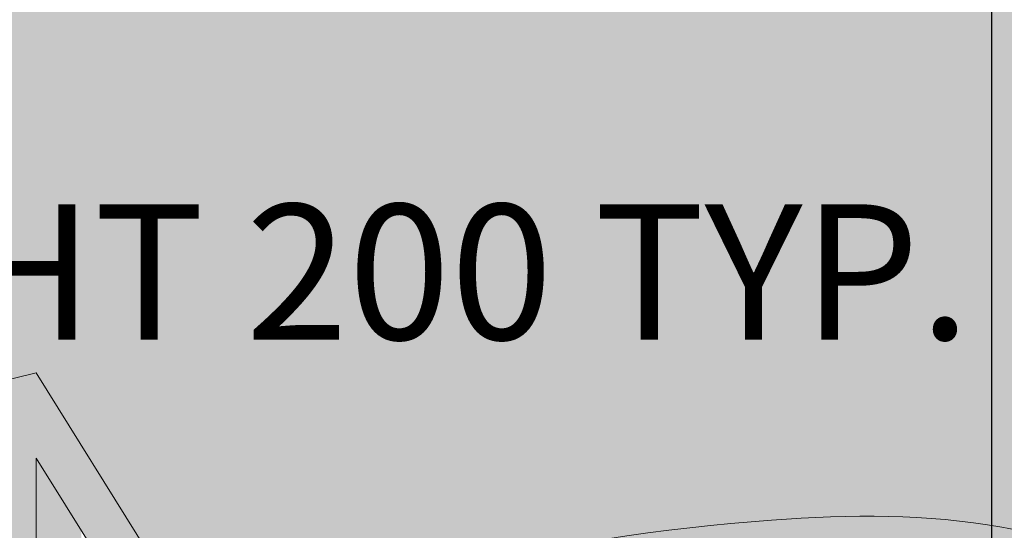
# Model space of a CAD drawing. Units: millimetres. Extents: x 11032 to 26788, y 3406 to 24505.
# Tile 56 of 78: x 15266 to 16358, y 16877 to 17443. Entities that reach past the tile are written whole.
import ezdxf

# ---------------------------------------------------------------- set-up
doc = ezdxf.new("R2010")
doc.units = ezdxf.units.MM
doc.header["$MEASUREMENT"] = 0
for name, color, linetype, lineweight in [('A-ANNO-DIMS', 2, 'Continuous', 18), ('A-GLAZ', 250, 'Continuous', 20), ('A-ROOF', 7, 'Continuous', 30), ('E-LITE', 7, 'Continuous', 18), ('E-LITE-PATT', 7, 'Continuous', 13)]:
    doc.layers.add(name, color=color, linetype=linetype, lineweight=lineweight)
for name, color, linetype, lineweight, true_color in [('A-GLAZ-FRAM-PATT', 250, 'Continuous', 13, 0x262627), ('A-ROOF-PATT', 9, 'Continuous', 13, 0xc7c8ca), ('A-WALL-INTR-PATT', 251, 'Continuous', 13, 0x6c6b6a)]:
    doc.layers.add(name, color=color, linetype=linetype, lineweight=lineweight, true_color=true_color)
doc.styles.get("Standard").update_dxf_attribs({"font": 'arial.ttf'})
doc.dimstyles.get("Standard").update_dxf_attribs({"dimtxt": 150, "dimasz": 100, "dimexe": 10, "dimexo": 5, "dimgap": 5, "dimtad": 0, "dimtih": 1, "dimtoh": 1, "dimdec": 0, "dimzin": 0, "dimdsep": 46, "dimtxsty": 'Standard', "dimcen": 0.09, "dimadec": 0, "dimazin": 0, "dimtfac": 1, "dimtdec": 0, "dimtofl": 0, "dimtmove": 0, "dimatfit": 3, "dimfxl": 1, "dimtolj": 1, "dimtzin": 0, "dimarcsym": 0})

# ---------------------------------------------------------------- blocks, each defined once
blk = doc.blocks.new('*D24')
at = {"layer": 'A-ANNO-DIMS', "color": 0, "lineweight": -2, "transparency": 16777216}
for p, q in [((13310.2, 17138), (13310.2, 17173)), ((13510.2, 17138), (13510.2, 17173)), ((13210.2, 17163), (13110.2, 17163)), ((13610.2, 17163), (13710.2, 17163))]:
    blk.add_line(p, q, dxfattribs=at)
at = {"layer": 'A-ANNO-DIMS', "color": 0, "transparency": 16777216}
for points in [[(13210.2, 17179.6), (13210.2, 17146.3), (13310.2, 17163)], [(13610.2, 17179.6), (13610.2, 17146.3), (13510.2, 17163)]]:
    blk.add_solid(points, dxfattribs=at)
at = {"layer": 'Defpoints', "color": 0, "transparency": 16777216}
for p in [(13510.2, 17163), (13310.2, 17133), (13510.2, 17133)]:
    blk.add_point(p, dxfattribs=at)
at = {"layer": 'A-ANNO-DIMS', "color": 0, "transparency": 16777216, "insert": (15077.8, 17163), "char_height": 150, "attachment_point": 5}
blk.add_mtext('\\A1;RECESSED LIGHT 200 TYP.', dxfattribs=at)
blk = doc.blocks.new('*D36')
at = {"layer": 'A-ANNO-DIMS', "color": 0, "lineweight": -2, "transparency": 16777216}
for p, q in [((12301.3, 17115.9), (12301.3, 24416.9)), ((25397.4, 4466.4), (25397.4, 24416.9)), ((12401.3, 24406.9), (18569.2, 24406.9)), ((25297.4, 24406.9), (19129.5, 24406.9))]:
    blk.add_line(p, q, dxfattribs=at)
at = {"layer": 'A-ANNO-DIMS', "color": 0, "transparency": 16777216}
for points in [[(12401.3, 24423.5), (12401.3, 24390.2), (12301.3, 24406.9)], [(25297.4, 24423.5), (25297.4, 24390.2), (25397.4, 24406.9)]]:
    blk.add_solid(points, dxfattribs=at)
at = {"layer": 'Defpoints', "color": 0, "transparency": 16777216}
for p in [(25397.4, 24406.9), (12301.3, 17110.9), (25397.4, 4461.4)]:
    blk.add_point(p, dxfattribs=at)
at = {"layer": 'A-ANNO-DIMS', "color": 0, "transparency": 16777216, "insert": (18849.3, 24406.9), "char_height": 150, "attachment_point": 5}
blk.add_mtext('\\A1;13096', dxfattribs=at)
blk = doc.blocks.new('*D37')
at = {"layer": 'A-ANNO-DIMS', "color": 0, "lineweight": -2, "transparency": 16777216}
for p, q in [((18087.7, 23450.4), (11334.8, 23450.4)), ((11344.8, 23350.4), (11344.8, 14037.5)), ((11344.8, 4561.4), (11344.8, 13874.3)), ((12927.7, 4461.4), (11334.8, 4461.4))]:
    blk.add_line(p, q, dxfattribs=at)
at = {"layer": 'A-ANNO-DIMS', "color": 0, "transparency": 16777216}
for points in [[(11328.1, 23350.4), (11361.4, 23350.4), (11344.8, 23450.4)], [(11328.1, 4561.4), (11361.4, 4561.4), (11344.8, 4461.4)]]:
    blk.add_solid(points, dxfattribs=at)
at = {"layer": 'Defpoints', "color": 0, "transparency": 16777216}
for p in [(11344.8, 23450.4), (18092.7, 23450.4), (12932.7, 4461.4)]:
    blk.add_point(p, dxfattribs=at)
at = {"layer": 'A-ANNO-DIMS', "color": 0, "transparency": 16777216, "insert": (11344.8, 13955.9), "char_height": 150, "attachment_point": 5}
blk.add_mtext('\\A1;18989', dxfattribs=at)
blk = doc.blocks.new('*D45')
at = {"layer": 'A-ANNO-DIMS', "color": 0, "lineweight": -2, "transparency": 16777216}
for p, q in [((13792.4, 18518.9), (26363.9, 18518.9)), ((26353.9, 18418.9), (26353.9, 17450.3)), ((26353.9, 16318.4), (26353.9, 17287)), ((22902.4, 16218.4), (26363.9, 16218.4))]:
    blk.add_line(p, q, dxfattribs=at)
at = {"layer": 'A-ANNO-DIMS', "color": 0, "transparency": 16777216}
for points in [[(26337.2, 18418.9), (26370.6, 18418.9), (26353.9, 18518.9)], [(26337.2, 16318.4), (26370.6, 16318.4), (26353.9, 16218.4)]]:
    blk.add_solid(points, dxfattribs=at)
at = {"layer": 'Defpoints', "color": 0, "transparency": 16777216}
for p in [(13787.4, 18518.9), (26353.9, 18518.9), (22897.4, 16218.4)]:
    blk.add_point(p, dxfattribs=at)
at = {"layer": 'A-ANNO-DIMS', "color": 0, "transparency": 16777216, "insert": (26353.9, 17368.7), "char_height": 150, "attachment_point": 5}
blk.add_mtext('\\A1;2300.5', dxfattribs=at)
blk = doc.blocks.new('*D57')
at = {"layer": 'A-ANNO-DIMS', "color": 0, "lineweight": -2, "transparency": 16777216}
for p, q in [((14994.7, 7266.4), (14994.7, 24416.9)), ((20894.7, 7266.4), (20894.7, 24416.9)), ((15094.7, 24406.9), (17716, 24406.9)), ((20794.7, 24406.9), (18173.4, 24406.9))]:
    blk.add_line(p, q, dxfattribs=at)
at = {"layer": 'A-ANNO-DIMS', "color": 0, "transparency": 16777216}
for points in [[(15094.7, 24423.5), (15094.7, 24390.2), (14994.7, 24406.9)], [(20794.7, 24423.5), (20794.7, 24390.2), (20894.7, 24406.9)]]:
    blk.add_solid(points, dxfattribs=at)
at = {"layer": 'Defpoints', "color": 0, "transparency": 16777216}
for p in [(20894.7, 24406.9), (14994.7, 7261.4), (20894.7, 7261.4)]:
    blk.add_point(p, dxfattribs=at)
at = {"layer": 'A-ANNO-DIMS', "color": 0, "transparency": 16777216, "insert": (17944.7, 24406.9), "char_height": 150, "attachment_point": 5}
blk.add_mtext('\\A1;5900', dxfattribs=at)
blk = doc.blocks.new('*D60')
at = {"layer": 'A-ANNO-DIMS', "color": 0, "lineweight": -2, "transparency": 16777216}
for p, q in [((14994.7, 7266.4), (14994.7, 24416.9)), ((16344.7, 7266.4), (16344.7, 24416.9)), ((15094.7, 24406.9), (15448, 24406.9)), ((16244.7, 24406.9), (15891.4, 24406.9))]:
    blk.add_line(p, q, dxfattribs=at)
at = {"layer": 'A-ANNO-DIMS', "color": 0, "transparency": 16777216}
for points in [[(15094.7, 24423.5), (15094.7, 24390.2), (14994.7, 24406.9)], [(16244.7, 24423.5), (16244.7, 24390.2), (16344.7, 24406.9)]]:
    blk.add_solid(points, dxfattribs=at)
at = {"layer": 'Defpoints', "color": 0, "transparency": 16777216}
for p in [(16344.7, 24406.9), (14994.7, 7261.4), (16344.7, 7261.4)]:
    blk.add_point(p, dxfattribs=at)
at = {"layer": 'A-ANNO-DIMS', "color": 0, "transparency": 16777216, "insert": (15669.7, 24406.9), "char_height": 150, "attachment_point": 5}
blk.add_mtext('\\A1;1350', dxfattribs=at)

msp = doc.modelspace()

# ---------------------------------------------------------------- hatches: boundary and pattern name
at = {"layer": 'A-GLAZ-FRAM-PATT'}
h = msp.add_hatch(color=256, dxfattribs=at)
edge = h.paths.add_edge_path()
edge.add_line((15284.393, 17051.32), (15084.393, 17001.32))
edge.add_line((15084.393, 17001.32), (15084.393, 15951.32))
edge.add_spline(control_points=[(15084.393, 15951.32), (15157.266, 15924.219), (15224.458, 15897.808), (15284.393, 15870.289)], knot_values=[511.94901044, 511.94901044, 511.94901044, 511.94901044, 697.37159794, 697.37159794, 697.37159794, 697.37159794], degree=3, periodic=0)
edge.add_line((15284.393, 15870.289), (15284.393, 17051.32))
edge = h.paths.add_edge_path()
edge.add_line((15659.393, 16354.387), (15459.393, 16675.629))
edge.add_line((15459.393, 16675.629), (15459.393, 15771.505))
edge.add_spline(control_points=[(15459.393, 15771.505), (15501.891, 15741.568), (15571.096, 15682.692), (15632.72, 15612.509), (15659.393, 15578.299)], knot_values=[905.064582, 905.064582, 905.064582, 905.064582, 1079.4682707, 1223.15843531, 1223.15843531, 1223.15843531, 1223.15843531], degree=3, periodic=0)
edge.add_line((15659.393, 15578.299), (15659.393, 16354.387))
h.paths.add_polyline_path([(15284.393, 17051.32), (15284.393, 16956.717), (15784.393, 16153.61), (15784.393, 16248.213)])
at = {"layer": 'A-ROOF-PATT'}
h = msp.add_hatch(color=256, dxfattribs=at)
edge = h.paths.add_edge_path()
edge.add_spline(control_points=[(17532.827, 17324.837), (17391.335, 17349.016), (16840.872, 17494.912), (16080.055, 18069.544), (14738.803, 18299.641), (13382.429, 18838.336), (12580.532, 17870.207), (12430.422, 17563.822)], knot_values=[2977.60279446, 2977.60279446, 2977.60279446, 2977.60279446, 3438.18406011, 4811.64630219, 5622.86754827, 7588.02881883, 8560.66857913, 8560.66857913, 8560.66857913, 8560.66857913], degree=3, periodic=0)
edge.add_spline(control_points=[(12430.422, 17563.822), (12437.904, 17573.36), (12445.386, 17582.899), (12452.869, 17592.437), (12452.869, 17592.438), (12452.869, 17592.438), (12452.869, 17592.438)], knot_values=[1408.56413798, 1408.56413798, 1408.56413798, 1408.56413798, 1444.85989, 1444.85989, 1444.85989, 1444.86011829, 1444.86011829, 1444.86011829, 1444.86011829], degree=3, periodic=0)
edge.add_spline(control_points=[(12452.869, 17592.438), (12555.432, 17723.185), (12736.557, 17929.686), (13044.86, 18114.643), (13219.943, 18189.644), (13299.92, 18220.646)], knot_values=[339.31824597, 339.31824597, 339.31824597, 339.31824597, 836.83499673, 1151.25129334, 1408.56413798, 1408.56413798, 1408.56413798, 1408.56413798], degree=3, periodic=0)
edge.add_spline(control_points=[(13299.92, 18220.646), (13299.998, 18220.689), (13300.077, 18220.732), (13319.738, 18231.488), (13339.24, 18241.402), (13388.645, 18264.703), (13418.466, 18277.069), (13478.019, 18298.648), (13507.751, 18307.861), (13544.561, 18317.488), (13551.584, 18319.245), (13558.612, 18320.924)], knot_values=[3783.89509717, 3783.89509717, 3783.89509717, 3783.89509717, 3784.1737101, 3784.1737101, 3853.4666747, 3853.4666747, 3960.24019172, 3960.24019172, 4067.01370874, 4067.01370874, 4092.17446487, 4092.17446487, 4092.17446487, 4092.17446487], degree=3, periodic=0)
edge.add_spline(control_points=[(13558.612, 18320.924), (13581.407, 18326.373), (13604.25, 18331.007), (13657.184, 18339.957), (13687.338, 18343.732), (13748.098, 18348.892), (13778.704, 18350.276), (13840.46, 18350.833), (13871.609, 18350.005), (13934.496, 18346.313), (13966.232, 18343.449), (14030.297, 18335.871), (14062.625, 18331.158), (14127.853, 18320.088), (14160.753, 18313.73), (14241.357, 18296.556), (14289.343, 18284.997), (14386.31, 18259.688), (14435.291, 18245.941), (14534.161, 18217.034), (14584.049, 18201.875), (14684.682, 18170.964), (14735.427, 18155.212), (14837.763, 18123.971), (14889.354, 18108.482), (14954.971, 18089.677), (14968.586, 18085.823), (14992.391, 18079.184), (15002.566, 18076.376), (15021.739, 18071.153), (15030.731, 18068.729), (15047.707, 18064.21), (15055.694, 18062.106), (15079.815, 18055.825), (15095.905, 18051.728), (15143.966, 18039.717), (15175.729, 18032.084), (15254.84, 18013.501), (15301.798, 18002.866), (15394.186, 17981.845), (15439.615, 17971.459), (15528.833, 17950.135), (15572.62, 17939.197), (15658.477, 17916.021), (15700.546, 17903.785), (15753.633, 17886.734), (15765.446, 17882.835), (15786.574, 17875.653), (15795.915, 17872.404), (15810.108, 17867.349), (15814.99, 17865.588), (15824.736, 17862.029), (15829.611, 17860.226), (15844.241, 17854.75), (15854.002, 17851.008), (15883.312, 17839.521), (15902.885, 17831.512), (15966.355, 17804.548), (16010.39, 17784.302), (16098.838, 17741.267), (16143.25, 17718.478), (16232.497, 17671.098), (16277.332, 17646.507), (16367.515, 17596.295), (16412.862, 17570.676), (16504.202, 17519.209), (16550.194, 17493.362), (16643.009, 17442.263), (16689.831, 17417.011), (16756.517, 17382.472), (16775.937, 17372.58), (16795.455, 17362.84)], knot_values=[4092.17446487, 4092.17446487, 4092.17446487, 4092.17446487, 4173.78722577, 4173.78722577, 4280.56074279, 4280.56074279, 4387.33425981, 4387.33425981, 4494.10777683, 4494.10777683, 4600.88129386, 4600.88129386, 4707.65481088, 4707.65481088, 4814.4283279, 4814.4283279, 4967.12624049, 4967.12624049, 5119.82415308, 5119.82415308, 5272.52206566, 5272.52206566, 5425.21997825, 5425.21997825, 5577.91789084, 5577.91789084, 5617.78533194, 5617.78533194, 5647.46484794, 5647.46484794, 5673.61102495, 5673.61102495, 5696.74760695, 5696.74760695, 5743.68189033, 5743.68189033, 5837.55045709, 5837.55045709, 5979.72610459, 5979.72610459, 6121.90175208, 6121.90175208, 6264.07739957, 6264.07739957, 6406.25304706, 6406.25304706, 6447.25858494, 6447.25858494, 6480.04208821, 6480.04208821, 6497.30770621, 6497.30770621, 6514.5733242, 6514.5733242, 6549.10456019, 6549.10456019, 6618.16703217, 6618.16703217, 6772.66101707, 6772.66101707, 6927.15500198, 6927.15500198, 7081.64898689, 7081.64898689, 7236.1429718, 7236.1429718, 7390.6369567, 7390.6369567, 7545.13094161, 7545.13094161, 7608.19928683, 7608.19928683, 7608.19928683, 7608.19928683], degree=3, periodic=0)
edge.add_spline(control_points=[(16795.455, 17362.84), (16814.335, 17349.456), (16832.897, 17336.263), (16873.225, 17307.197), (16894.778, 17291.386), (16936.221, 17259.941), (16956.11, 17244.308), (16993.863, 17213.094), (17011.726, 17197.514), (17041.993, 17169.265), (17054.791, 17156.601), (17078.762, 17131.225), (17089.933, 17118.516), (17110.618, 17092.991), (17120.131, 17080.178), (17130.17, 17065.264), (17131.487, 17063.277), (17133.77, 17059.776), (17134.746, 17058.261), (17136.69, 17055.205), (17137.657, 17053.668), (17140.539, 17049.025), (17142.438, 17045.89), (17148.068, 17036.367), (17151.732, 17029.859), (17163.03, 17008.788), (17170.335, 16993.646), (17184.087, 16961.978), (17190.534, 16945.453), (17202.562, 16911.165), (17208.142, 16893.402), (17218.448, 16856.821), (17223.173, 16838.003), (17231.801, 16799.51), (17235.705, 16779.837), (17241.533, 16746.739), (17243.676, 16733.5), (17247.718, 16706.37), (17249.608, 16692.472), (17252.066, 16672.69), (17252.761, 16666.875), (17254.1, 16655.226), (17254.744, 16649.4), (17256.596, 16631.917), (17257.727, 16620.254), (17260.823, 16585.238), (17262.489, 16561.858), (17266.551, 16488.654), (17267.658, 16438.661), (17267.349, 16375.228), (17267.193, 16362.07), (17266.95, 16348.891)], knot_values=[15.11304723, 15.11304723, 15.11304723, 15.11304723, 82.69951457, 82.69951457, 165.39902914, 165.39902914, 248.09854371, 248.09854371, 330.79805828, 330.79805828, 397.94194582, 397.94194582, 465.08583335, 465.08583335, 532.22972088, 532.22972088, 542.53374101, 542.53374101, 550.35681582, 550.35681582, 558.17989062, 558.17989062, 573.82604024, 573.82604024, 605.11833946, 605.11833946, 672.76406143, 672.76406143, 740.4097834, 740.4097834, 808.05550537, 808.05550537, 875.70122735, 875.70122735, 943.34694932, 943.34694932, 987.66134917, 987.66134917, 1033.41216123, 1033.41216123, 1052.38508762, 1052.38508762, 1071.35801402, 1071.35801402, 1109.30386682, 1109.30386682, 1185.19557241, 1185.19557241, 1346.44190265, 1346.44190265, 1388.55866312, 1388.55866312, 1388.55866312, 1388.55866312], degree=3, periodic=0)
edge.add_spline(control_points=[(17266.95, 16348.891), (17266.95, 16348.891), (17266.95, 16348.891), (17266.95, 16348.891), (17253.182, 15602.417), (17239.414, 14855.943), (17225.646, 14109.469)], knot_values=[1388.55866312, 1388.55866312, 1388.55866312, 1388.55866312, 1388.55896543, 1388.55896543, 1388.55896543, 3774.07676609, 3774.07676609, 3774.07676609, 3774.07676609], degree=3, periodic=0)
edge.add_spline(control_points=[(17225.646, 14109.469), (17226.198, 14109.827), (17226.748, 14110.185), (17242.065, 14120.191), (17255.956, 14130.116), (17274.422, 14144.286), (17279.609, 14148.386), (17284.686, 14152.511)], knot_values=[1926.3423968, 1926.3423968, 1926.3423968, 1926.3423968, 1927.31672898, 1927.31672898, 1953.51217613, 1953.51217613, 1964.07323478, 1964.07323478, 1964.07323478, 1964.07323478], degree=3, periodic=0)
edge.add_spline(control_points=[(17284.686, 14152.511), (17315.791, 14194.761), (17384.413, 14446.273), (17407.128, 14793.401), (17407.093, 15295.84), (17423.274, 15626.362), (17415.601, 15782.507)], knot_values=[0, 0, 0, 0, 163.25546741, 619.22967667, 1171.8624483, 1621.63555623, 1621.63555623, 1621.63555623, 1621.63555623], degree=3, periodic=0)
edge.add_spline(control_points=[(17415.601, 15782.507), (17438.21, 16077.57), (17410.495, 16533.484), (17390.893, 17030.649), (17301.082, 17169.349)], knot_values=[543.97847526, 543.97847526, 543.97847526, 543.97847526, 1452.98527668, 1960.01149261, 1960.01149261, 1960.01149261, 1960.01149261], degree=3, periodic=0)
edge.add_spline(control_points=[(17301.082, 17169.349), (17346.58, 17157.64), (17392.235, 17147.336), (17467.161, 17132.609), (17496.336, 17127.412), (17525.58, 17122.709)], knot_values=[8131.59393903, 8131.59393903, 8131.59393903, 8131.59393903, 8269.73492727, 8269.73492727, 8357.5016646, 8357.5016646, 8357.5016646, 8357.5016646], degree=3, periodic=0)
edge.add_line((17525.58, 17122.709), (17532.827, 17324.837))
edge = h.paths.add_edge_path(flags=17)
edge.add_spline(control_points=[(13340.537, 14602.706), (13316.172, 14726.456), (13323.666, 14932.342), (13637.836, 15081.117), (13863.248, 15171.051), (14002.1, 15224.503), (14058.539, 15244.876)], knot_values=[680.89318617, 680.89318617, 680.89318617, 680.89318617, 1033.47282894, 1337.40083264, 1604.72142636, 1784.29447217, 1784.29447217, 1784.29447217, 1784.29447217], degree=3, periodic=0)
edge.add_spline(control_points=[(14058.539, 15244.876), (14058.289, 15275.236), (14057.634, 15305.434), (14055.312, 15376.527), (14053.359, 15417.248), (14048.642, 15497.048), (14045.89, 15536.143), (14042.888, 15574.619)], knot_values=[6573.10654186, 6573.10654186, 6573.10654186, 6573.10654186, 6636.73300118, 6636.73300118, 6723.88905466, 6723.88905466, 6809.63287714, 6809.63287714, 6809.63287714, 6809.63287714], degree=3, periodic=0)
edge.add_spline(control_points=[(14042.888, 15574.619), (13546.54, 15403.221), (13074.735, 15143.241), (13277.36, 14695.339), (13340.537, 14602.706)], knot_values=[503.79257829, 503.79257829, 503.79257829, 503.79257829, 1728.17876056, 2051.34843998, 2051.34843998, 2051.34843998, 2051.34843998], degree=3, periodic=0)
h = msp.add_hatch(color=256, dxfattribs=at)
h.set_gradient(color1=(254, 234, 185), color2=(254, 204, 102), name='HEMISPHERICAL')
edge = h.paths.add_edge_path()
edge.add_line((15084.393, 17001.32), (15284.393, 17051.32))
edge.add_line((15284.393, 17051.32), (15470.537, 16752.334))
edge.add_spline(control_points=[(15470.537, 16752.334), (15683.311, 16831.508), (16106.827, 16912.335), (16625.609, 16876.997), (17083.498, 16357.78), (17257.801, 16180.113)], knot_values=[0, 0, 0, 0, 655.29363337, 1252.01578382, 1989.61628586, 1989.61628586, 1989.61628586, 1989.61628586], degree=3, periodic=0)
edge.add_spline(control_points=[(17257.801, 16180.113), (17260.851, 16236.372), (17263.9, 16292.632), (17266.95, 16348.891)], knot_values=[1132.9967717, 1132.9967717, 1132.9967717, 1132.9967717, 1198.04642249, 1198.04642249, 1198.04642249, 1198.04642249], degree=3, periodic=0)
edge.add_spline(control_points=[(17266.95, 16348.891), (17267.193, 16362.07), (17267.349, 16375.228), (17267.658, 16438.661), (17266.551, 16488.654), (17262.489, 16561.858), (17260.823, 16585.238), (17257.727, 16620.254), (17256.596, 16631.917), (17254.744, 16649.4), (17254.1, 16655.226), (17252.761, 16666.875), (17252.066, 16672.69), (17249.608, 16692.472), (17247.718, 16706.37), (17243.676, 16733.5), (17241.533, 16746.739), (17235.705, 16779.837), (17231.801, 16799.51), (17223.173, 16838.003), (17218.448, 16856.821), (17208.142, 16893.402), (17202.562, 16911.165), (17190.534, 16945.453), (17184.087, 16961.978), (17170.335, 16993.646), (17163.03, 17008.788), (17151.732, 17029.859), (17148.068, 17036.367), (17142.438, 17045.89), (17140.539, 17049.025), (17137.657, 17053.668), (17136.69, 17055.205), (17134.746, 17058.261), (17133.77, 17059.776), (17131.487, 17063.277), (17130.17, 17065.264), (17120.131, 17080.178), (17110.618, 17092.991), (17089.933, 17118.516), (17078.762, 17131.225), (17054.791, 17156.601), (17041.993, 17169.265), (17011.726, 17197.514), (16993.863, 17213.094), (16956.11, 17244.308), (16936.221, 17259.941), (16894.778, 17291.386), (16873.225, 17307.197), (16832.897, 17336.263), (16814.335, 17349.456), (16795.455, 17362.84)], knot_values=[15.11304723, 15.11304723, 15.11304723, 15.11304723, 57.2298077, 57.2298077, 218.47613793, 218.47613793, 294.36784353, 294.36784353, 332.31369632, 332.31369632, 351.28662272, 351.28662272, 370.25954912, 370.25954912, 416.01036118, 416.01036118, 460.32476103, 460.32476103, 527.970483, 527.970483, 595.61620497, 595.61620497, 663.26192694, 663.26192694, 730.90764891, 730.90764891, 798.55337089, 798.55337089, 829.84567011, 829.84567011, 845.49181972, 845.49181972, 853.31489453, 853.31489453, 861.13796933, 861.13796933, 871.44198947, 871.44198947, 938.585877, 938.585877, 1005.72976453, 1005.72976453, 1072.87365206, 1072.87365206, 1155.57316663, 1155.57316663, 1238.2726812, 1238.2726812, 1320.97219578, 1320.97219578, 1388.55866312, 1388.55866312, 1388.55866312, 1388.55866312], degree=3, periodic=0)
edge.add_spline(control_points=[(16795.455, 17362.84), (16775.937, 17372.58), (16756.517, 17382.472), (16689.831, 17417.011), (16643.009, 17442.263), (16550.194, 17493.362), (16504.202, 17519.209), (16412.862, 17570.676), (16367.515, 17596.295), (16277.332, 17646.507), (16232.497, 17671.098), (16143.25, 17718.478), (16098.838, 17741.267), (16010.39, 17784.302), (15966.355, 17804.548), (15902.885, 17831.512), (15883.312, 17839.521), (15854.002, 17851.008), (15844.241, 17854.75), (15829.611, 17860.226), (15824.736, 17862.029), (15814.99, 17865.588), (15810.108, 17867.349), (15795.915, 17872.404), (15786.574, 17875.653), (15765.446, 17882.835), (15753.633, 17886.734), (15700.546, 17903.785), (15658.477, 17916.021), (15572.62, 17939.197), (15528.833, 17950.135), (15439.615, 17971.459), (15394.186, 17981.845), (15301.798, 18002.866), (15254.84, 18013.501), (15175.729, 18032.084), (15143.966, 18039.717), (15095.905, 18051.728), (15079.815, 18055.825), (15055.694, 18062.106), (15047.707, 18064.21), (15030.731, 18068.729), (15021.739, 18071.153), (15002.566, 18076.376), (14992.391, 18079.184), (14968.586, 18085.823), (14954.971, 18089.677), (14889.354, 18108.482), (14837.763, 18123.971), (14735.427, 18155.212), (14684.682, 18170.964), (14584.049, 18201.875), (14534.161, 18217.034), (14435.291, 18245.941), (14386.31, 18259.688), (14289.343, 18284.997), (14241.357, 18296.556), (14160.753, 18313.73), (14127.853, 18320.088), (14062.625, 18331.158), (14030.297, 18335.871), (13966.232, 18343.449), (13934.496, 18346.313), (13871.609, 18350.005), (13840.46, 18350.833), (13778.704, 18350.276), (13748.098, 18348.892), (13687.338, 18343.732), (13657.184, 18339.957), (13604.25, 18331.007), (13581.407, 18326.373), (13558.612, 18320.924)], knot_values=[4092.17446487, 4092.17446487, 4092.17446487, 4092.17446487, 4155.24281009, 4155.24281009, 4309.736795, 4309.736795, 4464.2307799, 4464.2307799, 4618.72476481, 4618.72476481, 4773.21874972, 4773.21874972, 4927.71273463, 4927.71273463, 5082.20671953, 5082.20671953, 5151.26919151, 5151.26919151, 5185.8004275, 5185.8004275, 5203.0660455, 5203.0660455, 5220.33166349, 5220.33166349, 5253.11516676, 5253.11516676, 5294.12070464, 5294.12070464, 5436.29635213, 5436.29635213, 5578.47199962, 5578.47199962, 5720.64764711, 5720.64764711, 5862.82329461, 5862.82329461, 5956.69186137, 5956.69186137, 6003.62614475, 6003.62614475, 6026.76272675, 6026.76272675, 6052.90890376, 6052.90890376, 6082.58841976, 6082.58841976, 6122.45586086, 6122.45586086, 6275.15377345, 6275.15377345, 6427.85168604, 6427.85168604, 6580.54959862, 6580.54959862, 6733.24751121, 6733.24751121, 6885.9454238, 6885.9454238, 6992.71894082, 6992.71894082, 7099.49245784, 7099.49245784, 7206.26597487, 7206.26597487, 7313.03949189, 7313.03949189, 7419.81300891, 7419.81300891, 7526.58652593, 7526.58652593, 7608.19928683, 7608.19928683, 7608.19928683, 7608.19928683], degree=3, periodic=0)
edge.add_spline(control_points=[(13558.612, 18320.924), (13472.381, 18287.498), (13386.15, 18254.072), (13299.92, 18220.646), (13299.92, 18220.646), (13299.92, 18220.646), (13299.92, 18220.646)], knot_values=[61.88324569, 61.88324569, 61.88324569, 61.88324569, 339.3179746, 339.3179746, 339.3179746, 339.31824597, 339.31824597, 339.31824597, 339.31824597], degree=3, periodic=0)
edge.add_spline(control_points=[(13299.92, 18220.646), (13219.943, 18189.644), (13044.86, 18114.643), (12736.557, 17929.686), (12555.432, 17723.185), (12452.869, 17592.438)], knot_values=[339.31824597, 339.31824597, 339.31824597, 339.31824597, 596.63109061, 911.04738723, 1408.56413798, 1408.56413798, 1408.56413798, 1408.56413798], degree=3, periodic=0)
edge.add_spline(control_points=[(12452.869, 17592.438), (12452.869, 17592.438), (12452.869, 17592.438), (12452.869, 17592.437), (12445.386, 17582.899), (12437.904, 17573.36), (12430.422, 17563.822)], knot_values=[1408.56413798, 1408.56413798, 1408.56413798, 1408.56413798, 1408.56436627, 1408.56436627, 1408.56436627, 1444.86011829, 1444.86011829, 1444.86011829, 1444.86011829], degree=3, periodic=0)
edge.add_spline(control_points=[(12430.422, 17563.822), (12373.797, 17448.248), (12157.302, 16836.764), (12751.985, 16393.69), (13424.325, 15907.903), (14042.888, 15574.619)], knot_values=[0, 0, 0, 0, 366.89930338, 1975.59410824, 2977.60279446, 2977.60279446, 2977.60279446, 2977.60279446], degree=3, periodic=0)
edge.add_spline(control_points=[(14042.888, 15574.619), (14042.839, 15575.252), (14042.789, 15575.886), (14039.681, 15615.607), (14036.366, 15654.052), (14029.551, 15729.305), (14026.05, 15766.114), (14019.175, 15837.686), (14015.8, 15872.45), (13903.823, 16338.596)], knot_values=[6310.22615039, 6310.22615039, 6310.22615039, 6310.22615039, 6311.63838141, 6311.63838141, 6398.79443489, 6398.79443489, 6485.95048837, 6485.95048837, 6573.10654186, 6573.10654186, 6573.10654186, 6573.10654186], degree=3, periodic=0)
edge.add_spline(control_points=[(13903.823, 16338.596), (14237.315, 16236.889), (14456.623, 16167.555), (14614.196, 16115.84)], knot_values=[0, 0, 0, 0, 202.98534191, 202.98534191, 202.98534191, 202.98534191], degree=3, periodic=0)
edge.add_spline(control_points=[(14614.196, 16115.84), (14663.209, 16178.992), (14799.965, 16341.237), (14969.915, 16481.426), (15084.393, 16556.825)], knot_values=[2405.03450449, 2405.03450449, 2405.03450449, 2405.03450449, 2644.88269663, 3039.27072715, 3039.27072715, 3039.27072715, 3039.27072715], degree=3, periodic=0)
edge.add_line((15084.393, 16556.825), (15084.393, 17001.32))
h.paths.add_polyline_path([(14195.599, 17606.181, -1), (14395.599, 17606.181, -1)], flags=16)
h.paths.add_polyline_path([(13310.178, 17032.97, -1), (13510.178, 17032.97, -1)], flags=16)
at = {"layer": 'A-WALL-INTR-PATT'}
h = msp.add_hatch(color=256, dxfattribs=at)
edge = h.paths.add_edge_path()
edge.add_line((15334.393, 16876.406), (15284.393, 16956.717))
edge.add_line((15284.393, 16956.717), (15284.393, 15870.289))
edge.add_spline(control_points=[(15284.393, 15870.289), (15297.64, 15864.208), (15314.459, 15856.202), (15330.647, 15848.071), (15334.393, 15846.165)], knot_values=[697.37159794, 697.37159794, 697.37159794, 697.37159794, 738.35185821, 750.8383504, 750.8383504, 750.8383504, 750.8383504], degree=3, periodic=0)
edge.add_line((15334.393, 15846.165), (15334.393, 16876.406))
edge = h.paths.add_edge_path()
edge.add_line((15459.393, 16675.629), (15423.061, 16733.987))
edge.add_spline(control_points=[(15423.061, 16733.987), (15418.499, 16732.158), (15413.944, 16730.311), (15409.393, 16728.446)], knot_values=[2038.52225416, 2038.52225416, 2038.52225416, 2038.52225416, 2052.67140287, 2052.67140287, 2052.67140287, 2052.67140287], degree=3, periodic=0)
edge.add_line((15409.393, 16728.446), (15409.393, 15804.345))
edge.add_spline(control_points=[(15409.393, 15804.345), (15426.785, 15793.692), (15443.411, 15782.764), (15459.393, 15771.505)], knot_values=[839.47587364, 839.47587364, 839.47587364, 839.47587364, 905.064582, 905.064582, 905.064582, 905.064582], degree=3, periodic=0)
edge.add_line((15459.393, 15771.505), (15459.393, 16675.629))
edge = h.paths.add_edge_path()
edge.add_line((15709.393, 16274.076), (15659.393, 16354.387))
edge.add_line((15659.393, 16354.387), (15659.393, 15578.299))
edge.add_spline(control_points=[(15659.393, 15578.299), (15676.505, 15556.352), (15693.138, 15533.373), (15709.393, 15509.31)], knot_values=[1223.15843531, 1223.15843531, 1223.15843531, 1223.15843531, 1315.34242932, 1315.34242932, 1315.34242932, 1315.34242932], degree=3, periodic=0)
edge.add_line((15709.393, 15509.31), (15709.393, 16274.076))
at = {"layer": 'E-LITE-PATT'}
h = msp.add_hatch(color=256, dxfattribs=at)
edge = h.paths.add_edge_path()
edge.add_spline(control_points=[(15084.393, 16556.825), (14969.915, 16481.426), (14799.965, 16341.237), (14663.209, 16178.992), (14614.196, 16115.84)], knot_values=[2405.03450449, 2405.03450449, 2405.03450449, 2405.03450449, 2799.42253502, 3039.27072715, 3039.27072715, 3039.27072715, 3039.27072715], degree=3, periodic=0)
edge.add_spline(control_points=[(14614.196, 16115.84), (14650.957, 16103.776), (14684.357, 16092.67), (14715.064, 16082.336)], knot_values=[202.98534191, 202.98534191, 202.98534191, 202.98534191, 250.34086155, 250.34086155, 250.34086155, 250.34086155], degree=3, periodic=0)
edge.add_spline(control_points=[(14715.064, 16082.336), (14732.32, 16103.979), (14749.873, 16125.274), (14780.086, 16160.475), (14792.544, 16174.592), (14817.876, 16202.424), (14830.748, 16216.137), (14853.903, 16239.975), (14864.109, 16250.213), (14884.415, 16270.066), (14894.503, 16279.688), (14918.667, 16302.183), (14932.865, 16314.967), (14987.375, 16362.454), (15029.339, 16395.81), (15076.718, 16430.13), (15080.55, 16432.882), (15084.393, 16435.621)], knot_values=[2472.58550962, 2472.58550962, 2472.58550962, 2472.58550962, 2558.78653299, 2558.78653299, 2617.79751527, 2617.79751527, 2676.80849755, 2676.80849755, 2721.9976237, 2721.9976237, 2765.34243931, 2765.34243931, 2824.40593017, 2824.40593017, 2988.23517233, 2988.23517233, 3002.59878828, 3002.59878828, 3002.59878828, 3002.59878828], degree=3, periodic=0)
edge.add_line((15084.393, 16435.621), (15084.393, 16556.825))
edge = h.paths.add_edge_path()
edge.add_spline(control_points=[(17257.801, 16180.113), (17083.498, 16357.78), (16625.609, 16876.997), (16106.827, 16912.335), (15683.311, 16831.508), (15470.537, 16752.334)], knot_values=[0, 0, 0, 0, 737.60050204, 1334.32265249, 1989.61628586, 1989.61628586, 1989.61628586, 1989.61628586], degree=3, periodic=0)
edge.add_line((15470.537, 16752.334), (15524.528, 16665.613))
edge.add_spline(control_points=[(15524.528, 16665.613), (15525.367, 16665.915), (15526.207, 16666.217), (15585.74, 16687.58), (15645.217, 16705.796), (15751.033, 16733.457), (15797.417, 16743.949), (15889.17, 16761.791), (15934.539, 16769.141), (16001.164, 16777.942), (16023.135, 16780.505), (16055.649, 16783.812), (16066.413, 16784.825), (16082.439, 16786.212), (16087.761, 16786.652), (16098.362, 16787.489), (16103.645, 16787.886), (16113.574, 16788.594), (16118.22, 16788.91), (16129.942, 16789.661), (16136.98, 16790.07), (16160.862, 16791.296), (16177.385, 16791.865), (16209.759, 16792.279), (16225.609, 16792.125), (16256.756, 16790.981), (16272.053, 16789.992), (16302.249, 16787.067), (16317.147, 16785.133), (16346.731, 16780.197), (16361.418, 16777.195), (16390.79, 16769.979), (16405.476, 16765.764), (16435.066, 16755.942), (16449.97, 16750.334), (16480.199, 16737.514), (16495.524, 16730.301), (16518.956, 16718.108), (16526.841, 16713.814), (16542.775, 16704.739), (16550.823, 16699.959), (16563.039, 16692.397), (16567.144, 16689.805), (16577.49, 16683.149), (16583.769, 16678.999), (16606.897, 16663.324), (16624.116, 16650.909), (16664.382, 16620.344), (16687.634, 16601.588), (16734.666, 16561.798), (16758.449, 16540.764), (16811.484, 16492.225), (16840.771, 16464.327), (16898.924, 16407.388), (16927.79, 16378.347), (16976.921, 16328.12), (16997.415, 16306.918), (17037.673, 16265.01), (17057.437, 16244.305), (17096.046, 16203.842), (17114.892, 16184.084), (17151.499, 16145.947), (17169.261, 16127.569), (17186.418, 16110.081)], knot_values=[0, 0, 0, 0, 2.70856995, 2.70856995, 192.06253966, 192.06253966, 340.25443173, 340.25443173, 488.4463238, 488.4463238, 562.54226983, 562.54226983, 599.59024285, 599.59024285, 618.11422936, 618.11422936, 636.63821587, 636.63821587, 653.1204915, 653.1204915, 678.49014685, 678.49014685, 740.01795342, 740.01795342, 801.54575998, 801.54575998, 863.07356654, 863.07356654, 924.6013731, 924.6013731, 986.12917966, 986.12917966, 1047.65698622, 1047.65698622, 1109.18479279, 1109.18479279, 1170.71259935, 1170.71259935, 1201.47650263, 1201.47650263, 1232.24040591, 1232.24040591, 1247.62235755, 1247.62235755, 1270.70723576, 1270.70723576, 1331.82132989, 1331.82132989, 1411.19751033, 1411.19751033, 1490.57369076, 1490.57369076, 1587.69630201, 1587.69630201, 1684.81891326, 1684.81891326, 1755.8690587, 1755.8690587, 1826.91920415, 1826.91920415, 1897.96934959, 1897.96934959, 1969.01949503, 1969.01949503, 1969.01949503, 1969.01949503], degree=3, periodic=0)
edge.add_spline(control_points=[(17186.418, 16110.081), (17186.418, 16110.081), (17186.418, 16110.08), (17186.419, 16110.08), (17207.794, 16088.292), (17229.169, 16066.505), (17250.544, 16044.717)], knot_values=[-88.51855807, -88.51855807, -88.51855807, -88.51855807, -88.5172797, -88.5172797, -88.5172797, 0, 0, 0, 0], degree=3, periodic=0)
edge.add_spline(control_points=[(17250.544, 16044.717), (17251.307, 16059.803), (17252.131, 16075.51), (17253.018, 16091.882)], knot_values=[1232.05171003, 1232.05171003, 1232.05171003, 1232.05171003, 1250.98186159, 1250.98186159, 1250.98186159, 1250.98186159], degree=3, periodic=0)
edge.add_spline(control_points=[(17253.018, 16091.882), (17253.019, 16091.892), (17253.019, 16091.901), (17253.02, 16091.911), (17254.614, 16121.312), (17256.207, 16150.712), (17257.801, 16180.113)], knot_values=[1198.04642249, 1198.04642249, 1198.04642249, 1198.04642249, 1198.05760469, 1198.05760469, 1198.05760469, 1232.05171003, 1232.05171003, 1232.05171003, 1232.05171003], degree=3, periodic=0)

# ---------------------------------------------------------------- linework, layer by layer
at = {"layer": 'A-GLAZ'}
for p, q in [((15084.393, 17001.32), (15284.393, 17051.32)), ((15284.393, 17051.32), (16619.296, 14907.181)), ((15284.393, 15870.289), (15284.393, 16956.717)), ((15284.393, 16956.717), (16560.207, 14907.486))]:
    msp.add_line(p, q, dxfattribs=at)
at = {"layer": 'A-ROOF'}
for points, knots in [([(14042.888, 15574.619), (13424.325, 15907.903), (12751.985, 16393.69), (11963.048, 16981.495), (13249.687, 18891.056), (14738.803, 18299.641), (16080.055, 18069.544), (16966.203, 17400.251), (17654.208, 17293.942), (17944.704, 17286.735)], [0, 0, 0, 0, 1002.00868622, 2610.70349108, 3950.24255476, 5915.40382532, 6726.62507141, 8100.08731348, 8996.4318779, 8996.4318779, 8996.4318779, 8996.4318779]), ([(13299.92, 18220.646), (13299.998, 18220.689), (13300.077, 18220.732), (13319.738, 18231.488), (13339.24, 18241.402), (13388.645, 18264.703), (13418.466, 18277.069), (13478.019, 18298.648), (13507.751, 18307.861), (13567.331, 18323.443), (13597.18, 18329.812), (13657.184, 18339.957), (13687.338, 18343.732), (13748.098, 18348.892), (13778.704, 18350.276), (13840.46, 18350.833), (13871.609, 18350.005), (13934.496, 18346.313), (13966.232, 18343.449), (14030.297, 18335.871), (14062.625, 18331.158), (14127.853, 18320.088), (14160.753, 18313.73), (14241.357, 18296.556), (14289.343, 18284.997), (14386.31, 18259.688), (14435.291, 18245.941), (14534.161, 18217.034), (14584.049, 18201.875), (14684.682, 18170.964), (14735.427, 18155.212), (14837.763, 18123.971), (14889.354, 18108.482), (14954.971, 18089.677), (14968.586, 18085.823), (14992.391, 18079.184), (15002.566, 18076.376), (15021.739, 18071.153), (15030.731, 18068.729), (15047.707, 18064.21), (15055.694, 18062.106), (15079.815, 18055.825), (15095.905, 18051.728), (15143.966, 18039.717), (15175.729, 18032.084), (15254.84, 18013.501), (15301.798, 18002.866), (15394.186, 17981.845), (15439.615, 17971.459), (15528.833, 17950.135), (15572.62, 17939.197), (15658.477, 17916.021), (15700.546, 17903.785), (15753.633, 17886.734), (15765.446, 17882.835), (15786.574, 17875.653), (15795.915, 17872.404), (15810.108, 17867.349), (15814.99, 17865.588), (15824.736, 17862.029), (15829.611, 17860.226), (15844.241, 17854.75), (15854.002, 17851.008), (15883.312, 17839.521), (15902.885, 17831.512), (15966.355, 17804.548), (16010.39, 17784.302), (16098.838, 17741.267), (16143.25, 17718.478), (16232.497, 17671.098), (16277.332, 17646.507), (16367.515, 17596.295), (16412.862, 17570.676), (16504.202, 17519.209), (16550.194, 17493.362), (16643.009, 17442.263), (16689.831, 17417.011), (16756.517, 17382.472), (16775.937, 17372.58), (16795.455, 17362.84)], [3783.89509717, 3783.89509717, 3783.89509717, 3783.89509717, 3784.1737101, 3784.1737101, 3853.4666747, 3853.4666747, 3960.24019172, 3960.24019172, 4067.01370874, 4067.01370874, 4173.78722577, 4173.78722577, 4280.56074279, 4280.56074279, 4387.33425981, 4387.33425981, 4494.10777683, 4494.10777683, 4600.88129386, 4600.88129386, 4707.65481088, 4707.65481088, 4814.4283279, 4814.4283279, 4967.12624049, 4967.12624049, 5119.82415308, 5119.82415308, 5272.52206566, 5272.52206566, 5425.21997825, 5425.21997825, 5577.91789084, 5577.91789084, 5617.78533194, 5617.78533194, 5647.46484794, 5647.46484794, 5673.61102495, 5673.61102495, 5696.74760695, 5696.74760695, 5743.68189033, 5743.68189033, 5837.55045709, 5837.55045709, 5979.72610459, 5979.72610459, 6121.90175208, 6121.90175208, 6264.07739957, 6264.07739957, 6406.25304706, 6406.25304706, 6447.25858494, 6447.25858494, 6480.04208821, 6480.04208821, 6497.30770621, 6497.30770621, 6514.5733242, 6514.5733242, 6549.10456019, 6549.10456019, 6618.16703217, 6618.16703217, 6772.66101707, 6772.66101707, 6927.15500198, 6927.15500198, 7081.64898689, 7081.64898689, 7236.1429718, 7236.1429718, 7390.6369567, 7390.6369567, 7545.13094161, 7545.13094161, 7608.19928683, 7608.19928683, 7608.19928683, 7608.19928683])]:
    msp.add_open_spline(points, degree=3, knots=knots, dxfattribs=at)
at = {"layer": 'E-LITE'}
msp.add_open_spline([(17257.801, 16180.113), (17083.498, 16357.78), (16625.609, 16876.997), (16069.956, 16914.847), (15586.409, 16811.936), (15334.393, 16695.842)], degree=3, knots=[0, 0, 0, 0, 737.60050204, 1334.32265249, 2131.02016372, 2131.02016372, 2131.02016372, 2131.02016372], dxfattribs=at)

# ---------------------------------------------------------------- dimensions: what is measured, and where the dimension line sits
at = {"layer": 'A-ANNO-DIMS'}
for base, p1, p2, picture, middle in [((25397.404, 24406.858), (12301.265, 17110.885), (25397.404, 4461.399), '*D36', (18849.334, 24406.858)), ((20894.704, 24406.858), (14994.704, 7261.399), (20894.704, 7261.399), '*D57', (17944.704, 24406.858)), ((16344.704, 24406.858), (14994.704, 7261.399), (16344.704, 7261.399), '*D60', (15669.704, 24406.858))]:
    dim = msp.add_linear_dim(base=base, p1=p1, p2=p2, dimstyle='Standard', override={"dimdec": 0, "dimlfac": 1, "dimrnd": 0, "dimzin": 0, "dimdsep": 46, "dimlunit": 2}, dxfattribs=at)
    dim.commit()
    dim.dimension.update_dxf_attribs({"geometry": picture, "text_midpoint": middle})
for base, p1, p2, override, picture, middle in [((11344.765, 23450.358), (12932.665, 4461.399), (18092.739, 23450.358), {"dimdec": 0, "dimlfac": 1, "dimrnd": 0, "dimzin": 0, "dimdsep": 46, "dimlunit": 2}, '*D37', (11344.765, 13955.879)), ((26353.904, 18518.925), (22897.404, 16218.44), (13787.367, 18518.925), {"dimdec": 1, "dimlfac": 1, "dimrnd": 0, "dimzin": 0, "dimdsep": 46, "dimlunit": 2}, '*D45', (26353.904, 17368.682))]:
    dim = msp.add_linear_dim(base=base, p1=p1, p2=p2, angle=90, dimstyle='Standard', override=override, dxfattribs=at)
    dim.commit()
    dim.dimension.update_dxf_attribs({"geometry": picture, "text_midpoint": middle})
dim = msp.add_linear_dim(base=(13510.178, 17162.97), p1=(13310.178, 17132.97), p2=(13510.178, 17132.97), text='RECESSED LIGHT <> TYP.', dimstyle='Standard', override={"dimdec": 0, "dimlfac": 1, "dimrnd": 0, "dimzin": 0, "dimdsep": 46, "dimlunit": 2}, dxfattribs=at)
dim.commit()
dim.dimension.update_dxf_attribs({"geometry": '*D24', "text_midpoint": (15077.814, 17162.97)})

doc.saveas('drawing.dxf')
